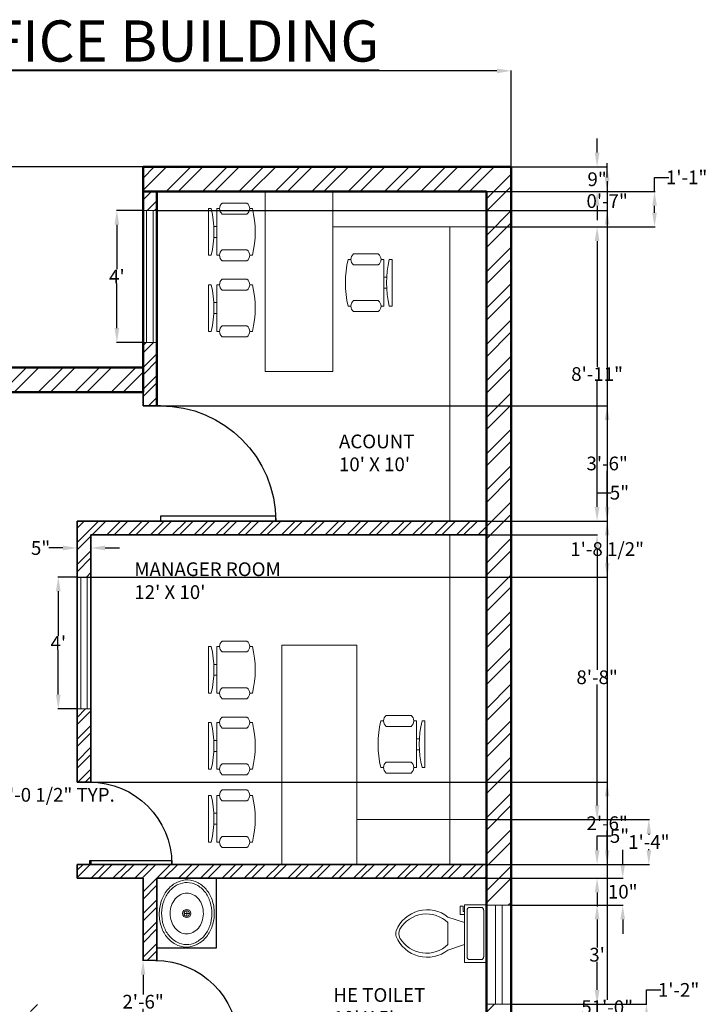
# Model space of a CAD drawing. Units: inches. Extents: x -355 to 263, y -871 to -163.
# Tile 6 of 6: x 10 to 260, y -521 to -163. Entities that reach past the tile are written whole.
import ezdxf

# ---------------------------------------------------------------- set-up
doc = ezdxf.new("R2010")
doc.units = ezdxf.units.IN
doc.header["$MEASUREMENT"] = 0
doc.layers.get('Defpoints').update_dxf_attribs({"color": 50})
for name, color, linetype, lineweight in [('A-ANNO-DIMS', 2, 'Continuous', 18), ('A-ANNO-TEXT', 7, 'Continuous', 25), ('A-AREA-IDEN', 7, 'Continuous', 18), ('A-FLOR-CASE', 9, 'Continuous', 25), ('A-FLOR-FIXT', 8, 'Continuous', 18), ('A-WALL-PATT', 252, 'Continuous', 13)]:
    doc.layers.add(name, color=color, linetype=linetype, lineweight=lineweight)
for name, color, linetype, lineweight, plot in [('CHAIR', 8, 'Continuous', 18, False), ('DOOR', 4, 'Continuous', 25, False), ('IWAL', 7, 'Continuous', 35, False), ('OWALL', 7, 'Continuous', 50, False), ('TABLE', 8, 'Continuous', 18, False), ('WIND', 3, 'Continuous', 18, False)]:
    doc.layers.add(name, color=color, linetype=linetype, lineweight=lineweight, plot=plot)
doc.styles.get("Standard").update_dxf_attribs({"font": 'arial.ttf'})
doc.dimstyles.get("Standard").update_dxf_attribs({"dimtxt": 5, "dimasz": 5.18, "dimexe": 0.18, "dimexo": 0.0625, "dimgap": 0.09, "dimtad": 0, "dimtih": 1, "dimtoh": 1, "dimdec": 0, "dimzin": 0, "dimdsep": 46, "dimlunit": 3, "dimtxsty": 'Standard', "dimcen": 0.09, "dimadec": 0, "dimazin": 0, "dimtfac": 1, "dimtdec": 0, "dimtofl": 0, "dimtmove": 0, "dimatfit": 3, "dimfxl": 1, "dimtolj": 1, "dimtzin": 0, "dimarcsym": 0})

# ---------------------------------------------------------------- blocks, each defined once
blk = doc.blocks.new('*U5')
for p, q in [((0, 0), (0, -6)), ((40, 0), (40, -6))]:
    blk.add_line(p, q)
blk.add_lwpolyline([(0, 0), (0, 40), (1.75, 40), (1.75, 0)], close=True)
blk.add_arc((0, 0), 40, 0, 90)
blk = doc.blocks.new('Toilet - top')
for p, q in [((9.5, -6), (9.5, -2)), ((-10, -8.5), (-8, -8.5)), ((-10, -9.5), (-10, -8.5)), ((-7, -9.5), (-10, -9.5)), ((-8, -8.5), (-8, -8)), ((-7, -8), (-7, -9.5)), ((-4, -8), (-6, -14)), ((4, -8), (6, -14)), ((4, -14), (-4, -14))]:
    blk.add_line(p, q)
blk.add_lwpolyline([(10.5, -8), (10.5, 0), (-10.5, 0), (-10.5, -8)], close=True)
for points in [[(-9.5, -2), (-9.5, -6)], [(8.5, -1), (-8.5, -1)], [(-8.5, -7), (8.5, -7)]]:
    blk.add_lwpolyline(points)
for centre, radius, start, end in [((-8.62, -1.88), 0.884, 81.8699, 188.1301), ((8.62, -1.88), 0.884, 351.8699, 98.1301), ((-8.62, -6.12), 0.884, 171.8699, 278.1301), ((8.62, -6.12), 0.884, 261.8699, 8.1301), ((3.52, -21.58), 12.17, 141.4691, 247.9714), ((4.2, -21.82), 11.33, 136.3677, 238.9468), ((-3.52, -21.58), 12.17, 292.0284, 38.5307), ((-4.2, -21.82), 11.33, 301.053, 43.6321), ((0, -27.88), 4, 245.7318, 294.2682), ((0, -29), 4, 254.8605, 285.1395)]:
    blk.add_arc(centre, radius, start, end)
blk = doc.blocks.new('Sink - Oval top')
for p, q in [((-1, 0), (1, 0)), ((0, 1), (0, -1))]:
    blk.add_line(p, q)
for points in [[(-12.23, 0.39, 0.117634), (-11.46, -3.36, 0.104469), (-8.88, -6.8, 0.090016), (-5.08, -9.07, 0.08192), (-0.32, -10.02, 0.08192), (4.49, -9.38, 0.090016), (8.42, -7.36, 0.104469), (11.22, -4.09, 0.117634), (12.23, -0.39, 0.117634), (11.46, 3.36, 0.104469), (8.88, 6.8, 0.090016), (5.08, 9.07, 0.08192), (0.32, 10.02, 0.08192), (-4.49, 9.38, 0.090016), (-8.42, 7.36, 0.104469), (-11.22, 4.09, 0.117634)], [(-11.29, 0.16, 0.118622), (-10.52, -3.25, 0.104678), (-8.07, -6.36, 0.089562), (-4.54, -8.37, 0.081185), (-0.13, -9.15, 0.081185), (4.3, -8.49, 0.089562), (7.89, -6.58, 0.104678), (10.42, -3.55, 0.118622), (11.29, -0.16, 0.118622), (10.52, 3.25, 0.104678), (8.07, 6.36, 0.089562), (4.54, 8.37, 0.081185), (0.13, 9.15, 0.081185), (-4.3, 8.49, 0.089562), (-7.89, 6.58, 0.104678), (-10.42, 3.55, 0.118622)], [(-7.42, 0.08, 0.118283), (-6.91, -2.17, 0.104607), (-5.29, -4.21, 0.089718), (-2.97, -5.53, 0.081436), (-0.07, -6.04, 0.081436), (2.84, -5.59, 0.089718), (5.2, -4.33, 0.104607), (6.86, -2.32, 0.118283), (7.42, -0.08, 0.118283), (6.91, 2.17, 0.104607), (5.29, 4.21, 0.089718), (2.97, 5.53, 0.081436), (0.07, 6.04, 0.081436), (-2.84, 5.59, 0.089718), (-5.2, 4.33, 0.104607), (-6.86, 2.32, 0.118283)]]:
    blk.add_lwpolyline(points, format="xyb", close=True)
for radius in [1.5, 1]:
    blk.add_circle((0, 0), radius)
blk = doc.blocks.new('Chair - Desk')
for p, q in [((-8.5, 0), (-8.5, -1)), ((-8.5, 0), (8.5, 0)), ((8.5, 0), (8.5, -1)), ((-8.5, -3), (-8.5, -4)), ((-8.5, -3), (8.5, -3)), ((-2, -3), (-2, -1.9355)), ((2, -1.9576), (2, -3)), ((8.5, -3), (8.5, -4)), ((-10.5, -5), (-10.5, -14)), ((-6.5, -14), (-6.5, -5)), ((6.5, -5), (6.5, -14)), ((10.5, -14), (10.5, -5)), ((-8.5, -15), (-8.5, -16)), ((8.5, -15), (8.5, -16))]:
    blk.add_line(p, q)
for centre, radius, start, end in [((0, 34.625), 36.625, 256.5803, 283.4197), ((-8.5, -6.5), 2.5, 36.8699, 143.1301), ((8.5, -6.5), 2.5, 36.8699, 143.1301), ((-8.5, -12.5), 2.5, 216.8699, 323.1301), ((8.5, -12.5), 2.5, 216.8699, 323.1301), ((0, 19.625), 36.625, 256.5803, 283.4197)]:
    blk.add_arc(centre, radius, start, end)
blk = doc.blocks.new('*D17')
at = {"layer": 'A-ANNO-DIMS', "color": 0, "lineweight": -2, "transparency": 16777216}
for p, q in [((54.62, -505.29), (54.5, -505.29)), ((54.68, -510.47), (54.68, -517.64)), ((54.68, -530.1), (54.68, -522.93)), ((54.74, -535.28), (54.86, -535.28))]:
    blk.add_line(p, q, dxfattribs=at)
at = {"layer": 'A-ANNO-DIMS', "color": 0, "lineweight": -3, "transparency": 16777216}
for points in [[(53.82, -510.47), (55.54, -510.47), (54.68, -505.29)], [(53.82, -530.1), (55.54, -530.1), (54.68, -535.28)]]:
    blk.add_solid(points, dxfattribs=at)
at = {"layer": 'Defpoints', "color": 0, "lineweight": -3, "transparency": 16777216}
for p in [(54.68, -505.29), (54.68, -505.29), (54.68, -535.28)]:
    blk.add_point(p, dxfattribs=at)
at = {"layer": 'A-ANNO-DIMS', "color": 0, "transparency": 16777216, "insert": (54.68, -520.28), "char_height": 5, "attachment_point": 5}
blk.add_mtext('\\A1;2\'-6"', dxfattribs=at)
blk = doc.blocks.new('*D19')
at = {"layer": 'A-ANNO-DIMS', "color": 0, "lineweight": -2, "transparency": 16777216}
for p, q in [((237.95, -521.16), (237.95, -515.98)), ((237.95, -515.98), (243.13, -515.98)), ((188.74, -521.16), (238.13, -521.16)), ((237.95, -530.1), (237.95, -526.34)), ((179.74, -535.28), (238.13, -535.28))]:
    blk.add_line(p, q, dxfattribs=at)
at = {"layer": 'A-ANNO-DIMS', "color": 0, "lineweight": -3, "transparency": 16777216}
for points in [[(237.09, -526.34), (238.81, -526.34), (237.95, -521.16)], [(237.09, -530.1), (238.81, -530.1), (237.95, -535.28)]]:
    blk.add_solid(points, dxfattribs=at)
at = {"layer": 'Defpoints', "color": 0, "lineweight": -3, "transparency": 16777216}
for p in [(188.68, -521.16), (237.95, -521.16), (179.68, -535.28)]:
    blk.add_point(p, dxfattribs=at)
at = {"layer": 'A-ANNO-DIMS', "color": 0, "transparency": 16777216, "insert": (249.63, -515.98), "char_height": 5, "attachment_point": 5}
blk.add_mtext('\\A1;1\'-2"', dxfattribs=at)
blk = doc.blocks.new('*D20')
at = {"layer": 'A-ANNO-DIMS', "color": 0, "lineweight": -2, "transparency": 16777216}
for p, q in [((188.74, -485.16), (220.15, -485.16)), ((219.97, -490.34), (219.97, -500.52)), ((219.97, -515.98), (219.97, -505.81)), ((188.74, -521.16), (220.15, -521.16))]:
    blk.add_line(p, q, dxfattribs=at)
at = {"layer": 'A-ANNO-DIMS', "color": 0, "lineweight": -3, "transparency": 16777216}
for points in [[(219.1, -490.34), (220.83, -490.34), (219.97, -485.16)], [(219.1, -515.98), (220.83, -515.98), (219.97, -521.16)]]:
    blk.add_solid(points, dxfattribs=at)
at = {"layer": 'Defpoints', "color": 0, "lineweight": -3, "transparency": 16777216}
for p in [(188.68, -485.16), (219.97, -485.16), (188.68, -521.16)]:
    blk.add_point(p, dxfattribs=at)
at = {"layer": 'A-ANNO-DIMS', "color": 0, "transparency": 16777216, "insert": (219.97, -503.16), "char_height": 5, "attachment_point": 5}
blk.add_mtext("\\A1;3'", dxfattribs=at)
blk = doc.blocks.new('*D21')
at = {"layer": 'A-ANNO-DIMS', "color": 0, "lineweight": -2, "transparency": 16777216}
for p, q in [((229.3, -470.1), (229.3, -464.92)), ((179.74, -475.28), (229.48, -475.28)), ((188.74, -485.16), (229.48, -485.16)), ((229.3, -490.34), (229.3, -495.52))]:
    blk.add_line(p, q, dxfattribs=at)
at = {"layer": 'A-ANNO-DIMS', "color": 0, "lineweight": -3, "transparency": 16777216}
for points in [[(228.43, -470.1), (230.16, -470.1), (229.3, -475.28)], [(228.43, -490.34), (230.16, -490.34), (229.3, -485.16)]]:
    blk.add_solid(points, dxfattribs=at)
at = {"layer": 'Defpoints', "color": 0, "lineweight": -3, "transparency": 16777216}
for p in [(179.68, -475.28), (229.3, -475.28), (188.68, -485.16)]:
    blk.add_point(p, dxfattribs=at)
at = {"layer": 'A-ANNO-DIMS', "color": 0, "transparency": 16777216, "insert": (229.3, -480.22), "char_height": 5, "attachment_point": 5}
blk.add_mtext('\\A1;10"', dxfattribs=at)
blk = doc.blocks.new('*D22')
at = {"layer": 'A-ANNO-DIMS', "color": 0, "lineweight": -2, "transparency": 16777216}
for p, q in [((219.97, -465.1), (219.97, -459.92)), ((219.97, -459.92), (225.15, -459.92)), ((179.74, -470.28), (220.15, -470.28)), ((179.74, -475.28), (220.15, -475.28)), ((219.97, -480.46), (219.97, -485.64))]:
    blk.add_line(p, q, dxfattribs=at)
at = {"layer": 'A-ANNO-DIMS', "color": 0, "lineweight": -3, "transparency": 16777216}
for points in [[(219.1, -465.1), (220.83, -465.1), (219.97, -470.28)], [(219.1, -480.46), (220.83, -480.46), (219.97, -475.28)]]:
    blk.add_solid(points, dxfattribs=at)
at = {"layer": 'Defpoints', "color": 0, "lineweight": -3, "transparency": 16777216}
for p in [(179.68, -470.28), (219.97, -470.28), (179.68, -475.28)]:
    blk.add_point(p, dxfattribs=at)
at = {"layer": 'A-ANNO-DIMS', "color": 0, "transparency": 16777216, "insert": (228.11, -459.92), "char_height": 5, "attachment_point": 5}
blk.add_mtext('\\A1;5"', dxfattribs=at)
blk = doc.blocks.new('*D23')
at = {"layer": 'A-ANNO-DIMS', "color": 0, "lineweight": -2, "transparency": 16777216}
for p, q in [((179.74, -453.97), (238.99, -453.97)), ((238.81, -459.15), (238.81, -459.53)), ((238.81, -465.1), (238.81, -464.73)), ((179.74, -470.28), (238.99, -470.28))]:
    blk.add_line(p, q, dxfattribs=at)
at = {"layer": 'A-ANNO-DIMS', "color": 0, "lineweight": -3, "transparency": 16777216}
for points in [[(237.95, -459.15), (239.67, -459.15), (238.81, -453.97)], [(237.95, -465.1), (239.67, -465.1), (238.81, -470.28)]]:
    blk.add_solid(points, dxfattribs=at)
at = {"layer": 'Defpoints', "color": 0, "lineweight": -3, "transparency": 16777216}
for p in [(179.68, -453.97), (238.81, -453.97), (179.68, -470.28)]:
    blk.add_point(p, dxfattribs=at)
at = {"layer": 'A-ANNO-DIMS', "color": 0, "transparency": 16777216, "insert": (238.81, -462.13), "char_height": 5, "attachment_point": 5}
blk.add_mtext('\\A1;1\'-4"', dxfattribs=at)
blk = doc.blocks.new('*D24')
at = {"layer": 'A-ANNO-DIMS', "color": 0, "lineweight": -2, "transparency": 16777216}
for p, q in [((179.74, -350.28), (220.15, -350.28)), ((219.97, -355.46), (219.97, -399.48)), ((219.97, -448.79), (219.97, -404.77)), ((179.74, -453.97), (220.15, -453.97))]:
    blk.add_line(p, q, dxfattribs=at)
at = {"layer": 'A-ANNO-DIMS', "color": 0, "lineweight": -3, "transparency": 16777216}
for points in [[(219.1, -355.46), (220.83, -355.46), (219.97, -350.28)], [(219.1, -448.79), (220.83, -448.79), (219.97, -453.97)]]:
    blk.add_solid(points, dxfattribs=at)
at = {"layer": 'Defpoints', "color": 0, "lineweight": -3, "transparency": 16777216}
for p in [(179.68, -350.28), (219.97, -350.28), (179.68, -453.97)]:
    blk.add_point(p, dxfattribs=at)
at = {"layer": 'A-ANNO-DIMS', "color": 0, "transparency": 16777216, "insert": (219.97, -402.13), "char_height": 5, "attachment_point": 5}
blk.add_mtext('\\A1;8\'-8"', dxfattribs=at)
blk = doc.blocks.new('*D25')
at = {"layer": 'A-ANNO-DIMS', "color": 0, "lineweight": -2, "transparency": 16777216}
for p, q in [((219.97, -340.1), (219.97, -334.92)), ((219.97, -334.92), (225.15, -334.92)), ((179.74, -345.28), (220.15, -345.28)), ((179.74, -350.28), (220.15, -350.28)), ((219.97, -355.46), (219.97, -360.64))]:
    blk.add_line(p, q, dxfattribs=at)
at = {"layer": 'A-ANNO-DIMS', "color": 0, "lineweight": -3, "transparency": 16777216}
for points in [[(219.1, -340.1), (220.83, -340.1), (219.97, -345.28)], [(219.1, -355.46), (220.83, -355.46), (219.97, -350.28)]]:
    blk.add_solid(points, dxfattribs=at)
at = {"layer": 'Defpoints', "color": 0, "lineweight": -3, "transparency": 16777216}
for p in [(179.68, -345.28), (219.97, -345.28), (179.68, -350.28)]:
    blk.add_point(p, dxfattribs=at)
at = {"layer": 'A-ANNO-DIMS', "color": 0, "transparency": 16777216, "insert": (228.11, -334.92), "char_height": 5, "attachment_point": 5}
blk.add_mtext('\\A1;5"', dxfattribs=at)
blk = doc.blocks.new('*D26')
at = {"layer": 'A-ANNO-DIMS', "color": 0, "lineweight": -2, "transparency": 16777216}
for p, q in [((179.74, -238.15), (220.15, -238.15)), ((219.97, -243.33), (219.97, -289.07)), ((219.97, -340.1), (219.97, -294.36)), ((179.74, -345.28), (220.15, -345.28))]:
    blk.add_line(p, q, dxfattribs=at)
at = {"layer": 'A-ANNO-DIMS', "color": 0, "lineweight": -3, "transparency": 16777216}
for points in [[(219.1, -243.33), (220.83, -243.33), (219.97, -238.15)], [(219.1, -340.1), (220.83, -340.1), (219.97, -345.28)]]:
    blk.add_solid(points, dxfattribs=at)
at = {"layer": 'Defpoints', "color": 0, "lineweight": -3, "transparency": 16777216}
for p in [(179.68, -238.15), (219.97, -238.15), (179.68, -345.28)]:
    blk.add_point(p, dxfattribs=at)
at = {"layer": 'A-ANNO-DIMS', "color": 0, "transparency": 16777216, "insert": (219.97, -291.72), "char_height": 5, "attachment_point": 5}
blk.add_mtext('\\A1;8\'-11"', dxfattribs=at)
blk = doc.blocks.new('*D27')
at = {"layer": 'A-ANNO-DIMS', "color": 0, "lineweight": -2, "transparency": 16777216}
for p, q in [((240.88, -225.28), (240.88, -220.1)), ((240.88, -220.1), (246.06, -220.1)), ((179.74, -225.28), (241.06, -225.28)), ((240.88, -232.97), (240.88, -230.46)), ((179.74, -238.15), (241.06, -238.15))]:
    blk.add_line(p, q, dxfattribs=at)
at = {"layer": 'A-ANNO-DIMS', "color": 0, "lineweight": -3, "transparency": 16777216}
for points in [[(240.01, -230.46), (241.74, -230.46), (240.88, -225.28)], [(240.01, -232.97), (241.74, -232.97), (240.88, -238.15)]]:
    blk.add_solid(points, dxfattribs=at)
at = {"layer": 'Defpoints', "color": 0, "lineweight": -3, "transparency": 16777216}
for p in [(179.68, -225.28), (240.88, -225.28), (179.68, -238.15)]:
    blk.add_point(p, dxfattribs=at)
at = {"layer": 'A-ANNO-DIMS', "color": 0, "transparency": 16777216, "insert": (252.56, -220.1), "char_height": 5, "attachment_point": 5}
blk.add_mtext('\\A1;1\'-1"', dxfattribs=at)
blk = doc.blocks.new('*D28')
at = {"layer": 'A-ANNO-DIMS', "color": 0, "lineweight": -2, "transparency": 16777216}
for p, q in [((219.97, -211.1), (219.97, -205.92)), ((188.74, -216.28), (220.15, -216.28)), ((179.74, -225.28), (220.15, -225.28)), ((219.97, -230.46), (219.97, -235.64))]:
    blk.add_line(p, q, dxfattribs=at)
at = {"layer": 'A-ANNO-DIMS', "color": 0, "lineweight": -3, "transparency": 16777216}
for points in [[(219.1, -211.1), (220.83, -211.1), (219.97, -216.28)], [(219.1, -230.46), (220.83, -230.46), (219.97, -225.28)]]:
    blk.add_solid(points, dxfattribs=at)
at = {"layer": 'Defpoints', "color": 0, "lineweight": -3, "transparency": 16777216}
for p in [(188.68, -216.28), (219.97, -216.28), (179.68, -225.28)]:
    blk.add_point(p, dxfattribs=at)
at = {"layer": 'A-ANNO-DIMS', "color": 0, "transparency": 16777216, "insert": (219.97, -220.78), "char_height": 5, "attachment_point": 5}
blk.add_mtext('\\A1;9"', dxfattribs=at)
blk = doc.blocks.new('*D45')
at = {"layer": 'A-ANNO-DIMS', "color": 0, "lineweight": -2, "transparency": 16777216}
for p, q in [((54.62, -232.18), (44.96, -232.18)), ((45.14, -237.36), (45.14, -253.59)), ((45.14, -275), (45.14, -258.77)), ((54.62, -280.18), (44.96, -280.18))]:
    blk.add_line(p, q, dxfattribs=at)
at = {"layer": 'A-ANNO-DIMS', "color": 0, "lineweight": -3, "transparency": 16777216}
for points in [[(44.28, -237.36), (46, -237.36), (45.14, -232.18)], [(44.28, -275), (46, -275), (45.14, -280.18)]]:
    blk.add_solid(points, dxfattribs=at)
at = {"layer": 'Defpoints', "color": 0, "lineweight": -3, "transparency": 16777216}
for p in [(45.14, -232.18), (54.68, -232.18), (54.68, -280.18)]:
    blk.add_point(p, dxfattribs=at)
at = {"layer": 'A-ANNO-DIMS', "color": 0, "transparency": 16777216, "insert": (45.14, -256.18), "char_height": 5, "attachment_point": 5}
blk.add_mtext("\\A1;4'", dxfattribs=at)
blk = doc.blocks.new('*D46')
at = {"layer": 'A-ANNO-DIMS', "color": 0, "lineweight": -2, "transparency": 16777216}
for p, q in [((30.62, -365.65), (23.63, -365.65)), ((23.81, -370.83), (23.81, -387.06)), ((23.81, -408.47), (23.81, -392.24)), ((30.62, -413.65), (23.63, -413.65))]:
    blk.add_line(p, q, dxfattribs=at)
at = {"layer": 'A-ANNO-DIMS', "color": 0, "lineweight": -3, "transparency": 16777216}
for points in [[(22.95, -370.83), (24.68, -370.83), (23.81, -365.65)], [(22.95, -408.47), (24.68, -408.47), (23.81, -413.65)]]:
    blk.add_solid(points, dxfattribs=at)
at = {"layer": 'Defpoints', "color": 0, "lineweight": -3, "transparency": 16777216}
for p in [(23.81, -365.65), (30.68, -365.65), (30.68, -413.65)]:
    blk.add_point(p, dxfattribs=at)
at = {"layer": 'A-ANNO-DIMS', "color": 0, "transparency": 16777216, "insert": (23.81, -389.65), "char_height": 5, "attachment_point": 5}
blk.add_mtext("\\A1;4'", dxfattribs=at)
blk = doc.blocks.new('*D47')
at = {"layer": 'A-ANNO-DIMS', "color": 0, "lineweight": -2, "transparency": 16777216}
for p, q in [((30.68, -350.34), (30.68, -355.24)), ((35.68, -350.34), (35.68, -355.24)), ((25.5, -355.06), (20.32, -355.06)), ((40.86, -355.06), (46.04, -355.06))]:
    blk.add_line(p, q, dxfattribs=at)
at = {"layer": 'A-ANNO-DIMS', "color": 0, "lineweight": -3, "transparency": 16777216}
for points in [[(25.5, -354.19), (25.5, -355.92), (30.68, -355.06)], [(40.86, -354.19), (40.86, -355.92), (35.68, -355.06)]]:
    blk.add_solid(points, dxfattribs=at)
at = {"layer": 'Defpoints', "color": 0, "lineweight": -3, "transparency": 16777216}
for p in [(30.68, -350.28), (35.68, -350.28), (30.68, -355.06)]:
    blk.add_point(p, dxfattribs=at)
at = {"layer": 'A-ANNO-DIMS', "color": 0, "transparency": 16777216, "insert": (17.36, -355.06), "char_height": 5, "attachment_point": 5}
blk.add_mtext('\\A1;5"', dxfattribs=at)
blk = doc.blocks.new('WIN-36IN-9IN-WALL')
for p, q in [((4.5, 36), (0, 36)), ((3.3, 36), (3.3, 0)), ((4.5, 36), (9, 36)), ((5.7, 36), (5.7, 0)), ((4.5, 0), (0, 0)), ((4.5, 0), (9, 0))]:
    blk.add_line(p, q)
blk = doc.blocks.new('WIN-48IN-5IN-WALL')
for p, q in [((2.5, 48), (0, 48)), ((1.3, 48), (1.3, 0)), ((2.5, 48), (5, 48)), ((3.7, 48), (3.7, 0)), ((2.5, 0), (0, 0)), ((2.5, 0), (5, 0))]:
    blk.add_line(p, q)
blk = doc.blocks.new('*D70')
at = {"layer": 'A-ANNO-DIMS', "color": 0, "lineweight": -2, "transparency": 16777216}
for p, q in [((-39.77, -436), (-39.77, -445.12)), ((-3.1, -436), (-3.1, -445.12)), ((-34.59, -444.94), (-8.28, -444.94)), ((-3.1, -444.94), (2.08, -444.94))]:
    blk.add_line(p, q, dxfattribs=at)
at = {"layer": 'A-ANNO-DIMS', "color": 0, "lineweight": -3, "transparency": 16777216}
for points in [[(-34.59, -444.07), (-34.59, -445.8), (-39.77, -444.94)], [(-8.28, -444.07), (-8.28, -445.8), (-3.1, -444.94)]]:
    blk.add_solid(points, dxfattribs=at)
at = {"layer": 'Defpoints', "color": 0, "lineweight": -3, "transparency": 16777216}
for p in [(-39.77, -435.94), (-3.1, -435.94), (-3.1, -444.94)]:
    blk.add_point(p, dxfattribs=at)
at = {"layer": 'A-ANNO-DIMS', "color": 0, "transparency": 16777216, "insert": (23.23, -444.94), "char_height": 5, "attachment_point": 5}
blk.add_mtext('\\A1;3\'-0 1/2" TYP.', dxfattribs=at)
blk = doc.blocks.new('*D75')
at = {"layer": 'A-ANNO-DIMS', "color": 0, "lineweight": -2, "transparency": 16777216}
for p, q in [((-301.32, -289.22), (-301.32, -181.15)), ((-296.14, -181.33), (-67.04, -181.33)), ((183.5, -181.33), (-45.6, -181.33)), ((188.68, -216.22), (188.68, -181.15))]:
    blk.add_line(p, q, dxfattribs=at)
at = {"layer": 'A-ANNO-DIMS', "color": 0, "lineweight": -3, "transparency": 16777216}
for points in [[(-296.14, -180.47), (-296.14, -182.19), (-301.32, -181.33)], [(183.5, -180.47), (183.5, -182.19), (188.68, -181.33)]]:
    blk.add_solid(points, dxfattribs=at)
at = {"layer": 'Defpoints', "color": 0, "lineweight": -3, "transparency": 16777216}
for p in [(188.68, -181.33), (188.68, -216.28), (-301.32, -289.28)]:
    blk.add_point(p, dxfattribs=at)
at = {"layer": 'A-ANNO-DIMS', "color": 0, "transparency": 16777216, "insert": (-56.32, -181.33), "char_height": 5, "attachment_point": 5}
blk.add_mtext('\\A1;40\'-10"', dxfattribs=at)
blk = doc.blocks.new('*D76')
at = {"layer": 'A-ANNO-DIMS', "color": 0, "lineweight": -2, "transparency": 16777216}
for p, q in [((188.74, -216.28), (223.81, -216.28)), ((223.63, -221.46), (223.63, -519.64)), ((223.63, -823.1), (223.63, -524.92)), ((188.74, -828.28), (223.81, -828.28))]:
    blk.add_line(p, q, dxfattribs=at)
at = {"layer": 'A-ANNO-DIMS', "color": 0, "lineweight": -3, "transparency": 16777216}
for points in [[(222.77, -221.46), (224.49, -221.46), (223.63, -216.28)], [(222.77, -823.1), (224.49, -823.1), (223.63, -828.28)]]:
    blk.add_solid(points, dxfattribs=at)
at = {"layer": 'Defpoints', "color": 0, "lineweight": -3, "transparency": 16777216}
for p in [(188.68, -216.28), (223.63, -216.28), (188.68, -828.28)]:
    blk.add_point(p, dxfattribs=at)
at = {"layer": 'A-ANNO-DIMS', "color": 0, "transparency": 16777216, "insert": (223.63, -522.28), "char_height": 5, "attachment_point": 5}
blk.add_mtext('\\A1;51\'-0"', dxfattribs=at)
blk = doc.blocks.new('*D77')
at = {"layer": 'A-ANNO-DIMS', "color": 0, "lineweight": -2, "transparency": 16777216}
for p, q in [((54.62, -216.28), (-336.45, -216.28)), ((-336.27, -221.46), (-336.27, -250.14)), ((-336.27, -284.1), (-336.27, -255.42)), ((54.62, -289.28), (-336.45, -289.28))]:
    blk.add_line(p, q, dxfattribs=at)
at = {"layer": 'A-ANNO-DIMS', "color": 0, "lineweight": -3, "transparency": 16777216}
for points in [[(-337.13, -221.46), (-335.41, -221.46), (-336.27, -216.28)], [(-337.13, -284.1), (-335.41, -284.1), (-336.27, -289.28)]]:
    blk.add_solid(points, dxfattribs=at)
at = {"layer": 'Defpoints', "color": 0, "lineweight": -3, "transparency": 16777216}
for p in [(-336.27, -216.28), (54.68, -216.28), (54.68, -289.28)]:
    blk.add_point(p, dxfattribs=at)
at = {"layer": 'A-ANNO-DIMS', "color": 0, "transparency": 16777216, "insert": (-336.27, -252.78), "char_height": 5, "attachment_point": 5}
blk.add_mtext('\\A1;6\'-1"', dxfattribs=at)
blk = doc.blocks.new('*D90')
at = {"layer": 'A-ANNO-DIMS', "color": 0, "lineweight": -2, "transparency": 16777216}
for p, q in [((30.74, -440.29), (223.81, -440.29)), ((223.63, -445.47), (223.63, -452.64)), ((223.63, -465.1), (223.63, -457.93)), ((30.74, -470.28), (223.81, -470.28))]:
    blk.add_line(p, q, dxfattribs=at)
at = {"layer": 'A-ANNO-DIMS', "color": 0, "lineweight": -3, "transparency": 16777216}
for points in [[(222.77, -445.47), (224.49, -445.47), (223.63, -440.29)], [(222.77, -465.1), (224.49, -465.1), (223.63, -470.28)]]:
    blk.add_solid(points, dxfattribs=at)
at = {"layer": 'Defpoints', "color": 0, "lineweight": -3, "transparency": 16777216}
for p in [(30.68, -440.29), (30.68, -470.28), (223.63, -470.28)]:
    blk.add_point(p, dxfattribs=at)
at = {"layer": 'A-ANNO-DIMS', "color": 0, "transparency": 16777216, "insert": (223.63, -455.28), "char_height": 5, "attachment_point": 5}
blk.add_mtext('\\A1;2\'-6"', dxfattribs=at)
blk = doc.blocks.new('*D91')
at = {"layer": 'A-ANNO-DIMS', "color": 0, "lineweight": -2, "transparency": 16777216}
for p, q in [((54.74, -303.28), (223.81, -303.28)), ((223.63, -308.46), (223.63, -321.64)), ((223.63, -340.1), (223.63, -326.92)), ((59.21, -345.28), (223.81, -345.28))]:
    blk.add_line(p, q, dxfattribs=at)
at = {"layer": 'A-ANNO-DIMS', "color": 0, "lineweight": -3, "transparency": 16777216}
for points in [[(222.77, -308.46), (224.49, -308.46), (223.63, -303.28)], [(222.77, -340.1), (224.49, -340.1), (223.63, -345.28)]]:
    blk.add_solid(points, dxfattribs=at)
at = {"layer": 'Defpoints', "color": 0, "lineweight": -3, "transparency": 16777216}
for p in [(54.68, -303.28), (59.14, -345.28), (223.63, -345.28)]:
    blk.add_point(p, dxfattribs=at)
at = {"layer": 'A-ANNO-DIMS', "color": 0, "transparency": 16777216, "insert": (223.63, -324.28), "char_height": 5, "attachment_point": 5}
blk.add_mtext('\\A1;3\'-6"', dxfattribs=at)
blk = doc.blocks.new('*D92')
at = {"layer": 'A-ANNO-DIMS', "color": 0, "lineweight": -2, "transparency": 16777216}
for p, q in [((223.63, -220.1), (223.63, -214.92)), ((59.74, -225.28), (223.81, -225.28)), ((59.74, -232.18), (223.81, -232.18)), ((223.63, -237.36), (223.63, -242.54))]:
    blk.add_line(p, q, dxfattribs=at)
at = {"layer": 'A-ANNO-DIMS', "color": 0, "lineweight": -3, "transparency": 16777216}
for points in [[(222.77, -220.1), (224.49, -220.1), (223.63, -225.28)], [(222.77, -237.36), (224.49, -237.36), (223.63, -232.18)]]:
    blk.add_solid(points, dxfattribs=at)
at = {"layer": 'Defpoints', "color": 0, "lineweight": -3, "transparency": 16777216}
for p in [(59.68, -225.28), (59.68, -232.18), (223.63, -232.18)]:
    blk.add_point(p, dxfattribs=at)
at = {"layer": 'A-ANNO-DIMS', "color": 0, "transparency": 16777216, "insert": (223.63, -228.73), "char_height": 5, "attachment_point": 5}
blk.add_mtext('\\A1;0\'-7"', dxfattribs=at)
blk = doc.blocks.new('*D93')
at = {"layer": 'A-ANNO-DIMS', "color": 0, "lineweight": -2, "transparency": 16777216}
for p, q in [((30.74, -345.28), (223.81, -345.28)), ((223.63, -350.46), (223.63, -352.79)), ((223.63, -360.47), (223.63, -358.14)), ((30.74, -365.65), (223.81, -365.65))]:
    blk.add_line(p, q, dxfattribs=at)
at = {"layer": 'A-ANNO-DIMS', "color": 0, "lineweight": -3, "transparency": 16777216}
for points in [[(222.77, -350.46), (224.49, -350.46), (223.63, -345.28)], [(222.77, -360.47), (224.49, -360.47), (223.63, -365.65)]]:
    blk.add_solid(points, dxfattribs=at)
at = {"layer": 'Defpoints', "color": 0, "lineweight": -3, "transparency": 16777216}
for p in [(30.68, -345.28), (30.68, -365.65), (223.63, -365.65)]:
    blk.add_point(p, dxfattribs=at)
at = {"layer": 'A-ANNO-DIMS', "color": 0, "transparency": 16777216, "insert": (223.63, -355.46), "char_height": 5, "attachment_point": 5}
blk.add_mtext('\\A1;1\'-8 1/2"', dxfattribs=at)

msp = doc.modelspace()

# ---------------------------------------------------------------- hatches: boundary and pattern name
at = {"layer": 'A-WALL-PATT'}
h = msp.add_hatch(dxfattribs=at)
h.set_pattern_fill('ANSI32', color=256, scale=25)
h.set_pattern_definition([(45, (-301.32, -828.28), (-6.62913, 6.62913), []), (45, (-296.9, -828.28), (-6.62913, 6.62913), [])])
h.paths.add_polyline_path([(54.68, -289.28), (-301.32, -289.28), (-301.32, -303.28), (-295.02, -303.28), (-292.32, -303.28), (-292.32, -298.28), (54.68, -298.28)])
h.paths.add_polyline_path([(188.68, -216.28), (54.68, -216.28), (54.68, -225.28), (179.68, -225.28), (179.68, -345.28), (179.68, -485.16), (184.18, -485.16), (188.68, -485.16)])
h.paths.add_polyline_path([(188.68, -521.16), (184.18, -521.16), (179.68, -521.16), (179.68, -540.28), (188.68, -540.28)])
h.paths.add_polyline_path([(164.68, -540.28), (155.68, -540.28), (155.68, -552.97), (160.18, -552.97), (164.68, -552.97)])
h.paths.add_polyline_path([(164.68, -588.97), (160.18, -588.97), (155.68, -588.97), (155.68, -620.04), (160.18, -620.04), (164.68, -620.04)])
h.paths.add_polyline_path([(164.68, -656.04), (160.18, -656.04), (155.68, -656.04), (155.68, -682.06), (160.18, -682.06), (164.68, -682.06)])
h.paths.add_polyline_path([(164.68, -718.06), (160.18, -718.06), (155.68, -718.06), (155.68, -730.28), (164.68, -730.28)])
h.paths.add_polyline_path([(188.68, -730.28), (179.68, -730.28), (179.68, -819.28), (73.9, -819.28), (73.9, -823.78), (73.9, -828.28), (188.68, -828.28)])
h.paths.add_polyline_path([(25.9, -819.28), (-41.45, -819.28), (-41.45, -823.78), (-41.45, -828.28), (25.9, -828.28), (25.9, -823.78)])
h.paths.add_polyline_path([(-113.45, -819.28), (-292.32, -819.28), (-292.32, -796.14), (-296.82, -796.14), (-301.32, -796.14), (-301.32, -828.28), (-113.45, -828.28), (-113.45, -823.78)])
h.paths.add_polyline_path([(-292.32, -480.28), (-292.32, -345.28), (-301.32, -345.28), (-301.32, -620.18), (-296.82, -620.18), (-292.32, -620.18)])
h.paths.add_polyline_path([(-292.32, -656.18), (-296.82, -656.18), (-301.32, -656.18), (-301.32, -700.14), (-296.82, -700.14), (-292.32, -700.14)])
h = msp.add_hatch(dxfattribs=at)
h.set_pattern_fill('ANSI32', color=256, scale=15)
h.set_pattern_definition([(45, (-292.3197, -819.28), (-3.977476, 3.977476), []), (45, (-289.668, -819.28), (-3.977476, 3.977476), [])])
h.paths.add_polyline_path([(59.68, -280.18), (57.18, -280.18), (54.68, -280.18), (54.68, -289.28), (54.68, -298.28), (54.68, -303.28), (59.68, -303.28)])
h.paths.add_polyline_path([(59.68, -225.28), (54.68, -225.28), (54.68, -232.18), (57.18, -232.18), (59.68, -232.18)])
h.paths.add_polyline_path([(18.68, -641.28), (18.68, -521.28), (13.68, -521.28), (13.68, -641.28), (-7.32, -665.28), (-105.32, -665.28), (-126.32, -641.28), (-126.32, -521.28), (-131.32, -521.28), (-131.32, -641.28), (-105.32, -670.28), (-7.32, -670.28)])
h.paths.add_polyline_path([(-167.32, -521.28), (-172.32, -521.28), (-172.32, -538.25), (-169.82, -538.25), (-167.32, -538.25)])
h.paths.add_polyline_path([(-134.32, -670.28), (-167.32, -670.28), (-167.32, -610.28), (-167.32, -586.25), (-169.82, -586.25), (-172.32, -586.25), (-172.32, -670.28), (-292.32, -670.28), (-292.32, -675.28), (-139.32, -675.28), (-134.32, -675.28)])
h.paths.add_polyline_path([(-167.32, -345.28), (-172.32, -345.28), (-172.32, -462.28), (-172.32, -480.28), (-292.32, -480.28), (-292.32, -485.28), (-172.32, -485.28), (-167.32, -485.28), (5.68, -485.28), (5.68, -480.28), (-167.32, -480.28)])
h.paths.add_polyline_path([(179.68, -345.28), (30.68, -345.28), (30.68, -365.65), (33.18, -365.65), (35.68, -365.65), (35.68, -350.28), (179.68, -350.28)])
h.paths.add_polyline_path([(-134.32, -707.28), (-139.32, -707.28), (-139.32, -819.28), (-134.32, -819.28)])
h.paths.add_polyline_path([(-9.32, -707.28), (-102.32, -707.28), (-102.32, -712.28), (-14.32, -712.28), (-14.32, -819.28), (-9.32, -819.28)])
h.paths.add_polyline_path([(179.68, -730.28), (22.68, -730.28), (22.68, -735.28), (179.68, -735.28)])
h.paths.add_polyline_path([(179.68, -470.28), (30.68, -470.28), (30.68, -475.28), (54.68, -475.28), (54.68, -505.29), (59.18, -505.29, -0.00418), (59.68, -505.29), (59.68, -475.28), (179.68, -475.28)])
h.paths.add_polyline_path([(35.68, -413.65), (33.18, -413.65), (30.68, -413.65), (30.68, -440.29), (35.18, -440.29, -0.00418), (35.68, -440.29)])
h.paths.add_polyline_path([(179.68, -535.28), (54.68, -535.28), (54.68, -540.28), (54.68, -570.29), (59.18, -570.29, -0.00418), (59.68, -570.29), (59.68, -540.28), (179.68, -540.28)])
h.paths.add_polyline_path([(121.93, -531.51), (160.73, -531.51), (160.73, -512.85), (121.93, -512.85)], flags=9)
h.paths.add_polyline_path([(49.47, -376.48), (111.2, -376.48), (111.2, -357.82), (49.47, -357.82)], flags=9)

# ---------------------------------------------------------------- linework, layer by layer
at = {"layer": 'A-FLOR-CASE'}
for p, q in [((81.29, -475.28), (81.29, -500.83)), ((81.29, -500.83), (59.68, -500.83))]:
    msp.add_line(p, q, dxfattribs=at)
at = {"layer": 'IWAL'}
for p, q in [((54.68, -298.28), (54.68, -303.28)), ((59.68, -303.28), (54.68, -303.28)), ((179.68, -345.28), (30.68, -345.28)), ((30.68, -345.28), (30.68, -440.29)), ((179.68, -350.28), (35.68, -350.28)), ((35.68, -350.28), (35.68, -440.29)), ((35.68, -468.97), (35.68, -470.28)), ((179.68, -470.28), (30.68, -470.28)), ((30.68, -470.28), (30.68, -475.28)), ((54.68, -475.28), (30.68, -475.28)), ((54.68, -475.28), (54.68, -505.29)), ((179.68, -475.28), (59.68, -475.28)), ((59.68, -475.28), (59.68, -505.29))]:
    msp.add_line(p, q, dxfattribs=at)
at = {"layer": 'OWALL'}
for p, q in [((54.68, -216.28), (188.68, -216.28)), ((54.68, -216.28), (54.68, -289.28)), ((188.68, -216.28), (188.68, -540.28)), ((54.68, -225.28), (179.68, -225.28)), ((59.68, -225.28), (59.68, -303.28)), ((179.68, -225.28), (179.68, -345.28)), ((54.68, -289.28), (-301.32, -289.28)), ((54.68, -298.28), (54.68, -289.28)), ((54.68, -298.28), (-292.32, -298.28)), ((179.68, -345.28), (179.68, -540.28))]:
    msp.add_line(p, q, dxfattribs=at)
at = {"layer": 'TABLE'}
for p, q in [((99.16, -225.28), (99.16, -290.84)), ((123.8, -290.84), (123.8, -225.28)), ((123.8, -238.15), (179.68, -238.15)), ((166.31, -238.15), (166.31, -345.28)), ((99.16, -290.84), (123.8, -290.84)), ((166.31, -350.28), (166.31, -470.28)), ((105.18, -470.28), (105.18, -390.4)), ((105.18, -390.4), (132.55, -390.4)), ((132.55, -390.4), (132.55, -470.28)), ((179.68, -453.97), (132.55, -453.97))]:
    msp.add_line(p, q, dxfattribs=at)

# ---------------------------------------------------------------- block references
at = {"layer": 'A-FLOR-FIXT'}
for name, p, rotation in [('Sink - Oval top', (70.59, -488.16), 90), ('Toilet - top', (179.68, -495.46), 269.9999999999998)]:
    msp.add_blockref(name, p, dxfattribs=dict(at, rotation=rotation))
at = {"layer": 'CHAIR'}
for p, rotation in [((78.5, -239.98), 90), ((145.32, -258.49), 270), ((78.5, -267.69), 90), ((78.5, -399.43), 90), ((78.5, -427.13), 90), ((157.23, -426.52), 270), ((78.5, -453.63), 90)]:
    msp.add_blockref('Chair - Desk', p, dxfattribs=dict(at, rotation=rotation))
at = {"layer": 'DOOR', "rotation": 270}
for p, xscale, yscale, zscale in [((60.98, -345.28), -1.049999999999999, 1.049999999999999, 1.049999999999999), ((35.18, -470.28), -0.7497657348060921, 0.7497657348060921, 0.7497657348060921), ((59.18, -535.28), -0.7497657348060921, 0.7497657348060921, 0.7497657348060921)]:
    msp.add_blockref('*U5', p, dxfattribs=dict(at, xscale=xscale, yscale=yscale, zscale=zscale))
at = {"layer": 'WIND'}
for name, p in [('WIN-48IN-5IN-WALL', (54.68, -280.18)), ('WIN-48IN-5IN-WALL', (30.68, -413.65)), ('WIN-36IN-9IN-WALL', (179.68, -521.16))]:
    msp.add_blockref(name, p, dxfattribs=at)

# ---------------------------------------------------------------- texts
at = {"layer": 'A-ANNO-TEXT', "insert": (-131.06, -162.96), "char_height": 15, "attachment_point": 1}
msp.add_mtext_dynamic_manual_height_columns('{\\fArial|b1|i0|c0|p34;\\LPLAN OF A OFFICE BUILDING}', width=417.8492, gutter_width=1, heights=[0], dxfattribs=at)
at = {"layer": 'A-AREA-IDEN', "char_height": 5, "attachment_point": 1}
for s, width, insert in [("{ACOUNT\\P10' X 10'}", 47.6588, (125.98, -313.76)), ("{MANAGER ROOM\\P12' X 10'}", 77.971, (51.48, -360.3)), ("{HE TOILET\\P10' X 5'}", 50.5823, (123.95, -515.34))]:
    msp.add_mtext_dynamic_manual_height_columns(s, width=width, gutter_width=1, heights=[0], dxfattribs=dict(at, insert=insert))

# ---------------------------------------------------------------- dimensions: what is measured, and where the dimension line sits
at = {"layer": 'A-ANNO-DIMS'}
for base, p1, p2, override, picture, middle in [((188.68, -181.33), (-301.32, -289.28), (188.68, -216.28), {"dimdec": 1, "dimlfac": 1, "dimrnd": 0, "dimzin": 1, "dimdsep": 46, "dimlunit": 4, "dimfrac": 2}, '*D75', (-56.32, -181.33)), ((30.68, -355.06), (35.68, -350.28), (30.68, -350.28), {"dimclrd": 0, "dimclre": 0, "dimclrt": 0}, '*D47', (17.36, -355.06))]:
    dim = msp.add_linear_dim(base=base, p1=p1, p2=p2, dimstyle='Standard', override=override, dxfattribs=at)
    dim.commit()
    dim.dimension.update_dxf_attribs({"geometry": picture, "text_midpoint": middle})
for base, p1, p2, angle, override, picture, middle in [((219.97, -216.28), (179.68, -225.28), (188.68, -216.28), 270, {"dimclrd": 0, "dimclre": 0, "dimclrt": 0}, '*D28', (219.97, -220.78)), ((223.63, -232.18), (59.68, -225.28), (59.68, -232.18), 90, {"dimdec": 1, "dimlfac": 1, "dimrnd": 0, "dimzin": 1, "dimdsep": 46, "dimlunit": 4, "dimfrac": 2}, '*D92', (223.63, -228.73)), ((-336.27, -216.28), (54.68, -289.28), (54.68, -216.28), 90, {"dimdec": 1, "dimlfac": 1, "dimrnd": 0, "dimzin": 1, "dimdsep": 46, "dimlunit": 4, "dimfrac": 2}, '*D77', (-336.27, -252.78)), ((240.88, -225.28), (179.68, -238.15), (179.68, -225.28), 270, {"dimclrd": 0, "dimclre": 0, "dimclrt": 0}, '*D27', (252.56, -220.1)), ((223.63, -216.28), (188.68, -828.28), (188.68, -216.28), 90, {"dimdec": 1, "dimlfac": 1, "dimrnd": 0, "dimzin": 1, "dimdsep": 46, "dimlunit": 4, "dimfrac": 2}, '*D76', (223.63, -522.28)), ((45.14, -232.18), (54.68, -280.18), (54.68, -232.18), 90, {"dimclrd": 0, "dimclre": 0, "dimclrt": 0}, '*D45', (45.14, -256.18)), ((219.97, -238.15), (179.68, -345.28), (179.68, -238.15), 270, {"dimclrd": 0, "dimclre": 0, "dimclrt": 0}, '*D26', (219.97, -291.72)), ((223.63, -345.28), (54.68, -303.28), (59.14, -345.28), 90, {"dimdec": 1, "dimlfac": 1, "dimrnd": 0, "dimzin": 1, "dimdsep": 46, "dimlunit": 4, "dimfrac": 2}, '*D91', (223.63, -324.28)), ((219.97, -345.28), (179.68, -350.28), (179.68, -345.28), 270, {"dimclrd": 0, "dimclre": 0, "dimclrt": 0}, '*D25', (228.11, -334.92)), ((223.63, -365.65), (30.68, -345.28), (30.68, -365.65), 90, {"dimdec": 1, "dimlfac": 1, "dimrnd": 0, "dimzin": 1, "dimdsep": 46, "dimlunit": 4, "dimfrac": 2}, '*D93', (223.63, -355.46)), ((219.97, -350.28), (179.68, -453.97), (179.68, -350.28), 270, {"dimclrd": 0, "dimclre": 0, "dimclrt": 0}, '*D24', (219.97, -402.13)), ((23.81, -365.65), (30.68, -413.65), (30.68, -365.65), 90, {"dimclrd": 0, "dimclre": 0, "dimclrt": 0}, '*D46', (23.81, -389.65)), ((223.63, -470.28), (30.68, -440.29), (30.68, -470.28), 90, {"dimdec": 1, "dimlfac": 1, "dimrnd": 0, "dimzin": 1, "dimdsep": 46, "dimlunit": 4, "dimfrac": 2}, '*D90', (223.63, -455.28)), ((219.97, -470.28), (179.68, -475.28), (179.68, -470.28), 270, {"dimclrd": 0, "dimclre": 0, "dimclrt": 0}, '*D22', (228.11, -459.92)), ((219.97, -485.16), (188.68, -521.16), (188.68, -485.16), 270, {"dimclrd": 0, "dimclre": 0, "dimclrt": 0}, '*D20', (219.97, -503.16)), ((54.68, -505.29), (54.68, -535.28), (54.68, -505.29), 90, {"dimclrd": 0, "dimclre": 0, "dimclrt": 0}, '*D17', (54.68, -520.28)), ((237.95, -521.16), (179.68, -535.28), (188.68, -521.16), 270, {"dimclrd": 0, "dimclre": 0, "dimclrt": 0}, '*D19', (249.63, -515.98))]:
    dim = msp.add_linear_dim(base=base, p1=p1, p2=p2, angle=angle, dimstyle='Standard', override=override, dxfattribs=at)
    dim.commit()
    dim.dimension.update_dxf_attribs({"geometry": picture, "text_midpoint": middle})
dim = msp.add_linear_dim(base=(-3.1, -444.94), p1=(-39.77, -435.94), p2=(-3.1, -435.94), text='<> TYP.', dimstyle='Standard', override={"dimdec": 1, "dimlfac": 1, "dimrnd": 0, "dimzin": 1, "dimdsep": 46, "dimlunit": 4, "dimfrac": 2}, dxfattribs=at)
dim.commit()
dim.dimension.update_dxf_attribs({"geometry": '*D70', "text_midpoint": (23.23, -444.94)})
for base, p1, p2, picture, middle in [((238.81, -453.97), (179.68, -470.28), (179.68, -453.97), '*D23', (238.81, -462.13)), ((229.3, -475.28), (188.68, -485.16), (179.68, -475.28), '*D21', (229.3, -480.22))]:
    dim = msp.add_linear_dim(base=base, p1=p1, p2=p2, angle=270, dimstyle='Standard', override={"dimclrd": 0, "dimclre": 0, "dimclrt": 0}, dxfattribs=at)
    dim.commit()
    dim.dimension.update_dxf_attribs({"geometry": picture, "text_midpoint": middle, "dimtype": 160})

doc.saveas('drawing.dxf')
